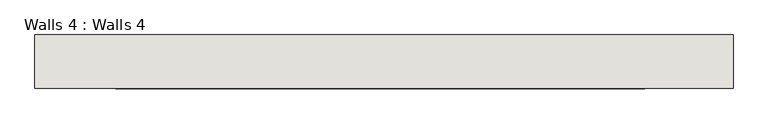
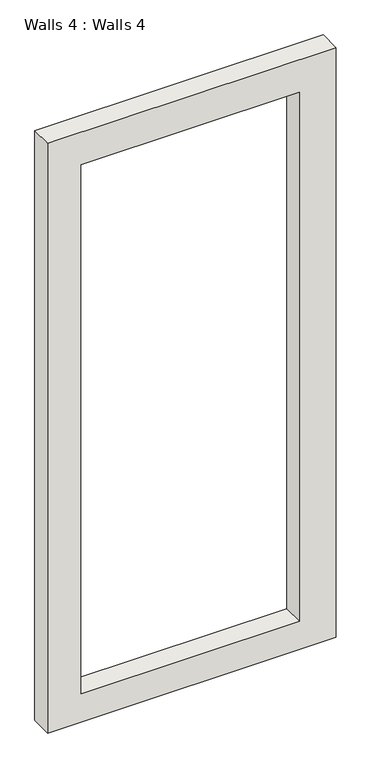
"""IFC4 building model written with IfcOpenShell, lengths in millimetres: wall geometry, Walls 4 : Walls 4."""

from ifc_helpers import new_model, si_unit, frame, origin, place, context, project, spatial, polyline, outline, extrude, source, transform, mapped, element, save


def walls_4_walls_4_f4f7f16f(model_context):
    return source(origin(), model_context, "Body", "SweptSolid", [
        extrude(outline(polyline([(6289.8374945, -4650.6320452), (6289.8374945, -7190.6320452), (803.4374945, -7190.6320452), (803.4374945, -4650.6320452), (6289.8374945, -4650.6320452)]), holes=[polyline([(5988.5853432, -4972.3150386), (1066.8, -4972.3150386), (1066.8, -6896.7101003), (5988.5853432, -6896.7101003), (5988.5853432, -4972.3150386)])]), frame((0.0, -4567.3270129, 0.0), z_axis=(0.0, 1.0, 0.0), x_axis=(0.0, 0.0, 1.0)), (0.0, 0.0, 1.0), 194.9163373),
    ])


if __name__ == "__main__":
    model = new_model("IFC4")
    model_context = context("Model", 3, world=origin())
    ifc_project = project(units=[si_unit("LENGTHUNIT", "METRE", prefix="MILLI")], contexts=[model_context])
    site = spatial("IfcSite", under=ifc_project)
    building = spatial("IfcBuilding", under=site)
    placement = place(None, origin())
    walls_4_walls_4_shape = walls_4_walls_4_f4f7f16f(model_context)
    element("IfcWall", 1, ObjectType="Walls 4 : Walls 4", at=placement, inside=building, context=model_context, shape_type="MappedRepresentation", body=[
        mapped(walls_4_walls_4_shape, transform((0.0, 0.0, 0.0), x_axis=(1.0, 0.0, 0.0), y_axis=(0.0, 1.0, 0.0), z_axis=(0.0, 0.0, 1.0))),
    ])
    save(model, "model.ifc")

# Revit data of these elements
# Element 1 (IfcWall, "Walls 4 : Walls 4")
#   Materials on its faces: "Default Wall"
# Materials
#   "Default Wall": colour RGB 128 128 128, transparency 0
